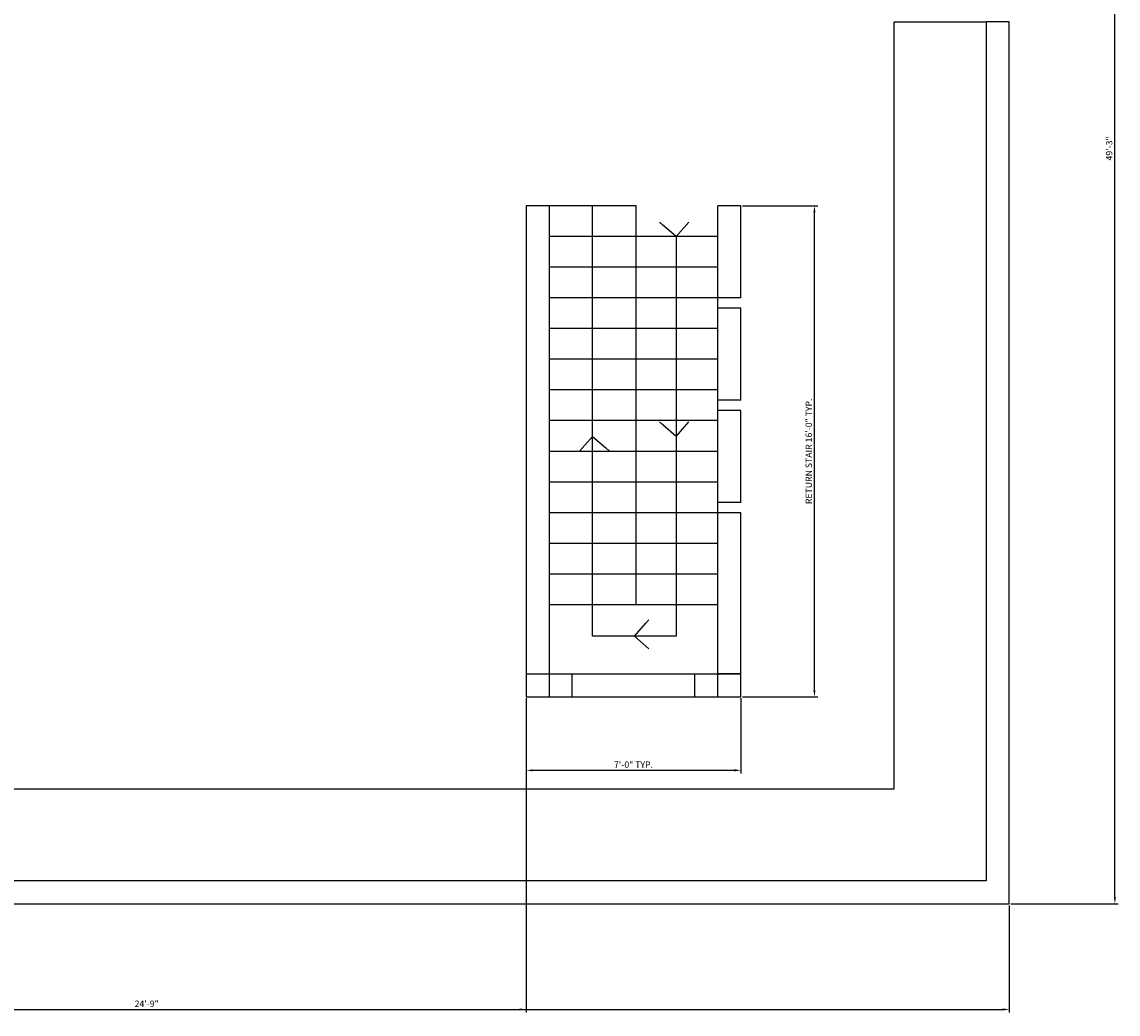
# Model space of a CAD drawing. Units: inches. Extents: x 250205121 to 250208111, y 89832590 to 89833271.
# Tile 3 of 14: x 250205601 to 250206030, y 89832590 to 89832978. Entities that reach past the tile are written whole.
import ezdxf

# ---------------------------------------------------------------- set-up
doc = ezdxf.new("R2010")
doc.units = ezdxf.units.IN
for name, color, linetype, lineweight in [('A-FLOR-STRS', 7, 'Continuous', 25), ('C-PROP', 8, 'Continuous', 25), ('dimensions', 2, 'Continuous', 18)]:
    doc.layers.add(name, color=color, linetype=linetype, lineweight=lineweight)
doc.styles.get("Standard").update_dxf_attribs({"font": 'arial.ttf'})
doc.dimstyles.new('ISO-25', dxfattribs={"dimtxt": 2.5, "dimasz": 2.5, "dimexe": 1.25, "dimexo": 0.625, "dimtad": 1, "dimlunit": 4, "dimtxsty": 'Standard', "dimcen": 2.5, "dimadec": 0, "dimazin": 0, "dimtfac": 1, "dimtmove": 0, "dimatfit": 3, "dimfxl": 1, "dimarcsym": 0})

# ---------------------------------------------------------------- blocks, each defined once
blk = doc.blocks.new('STAIR-RETURN')
for p, q in [((9, 192), (0, 192)), ((0, 192), (0, 0)), ((43, 192), (9, 192)), ((9, 192), (9, 0)), ((26, 23.7), (26, 192)), ((43, 36), (43, 192)), ((84, 192), (75, 192)), ((75, 0), (75, 192)), ((84, 156), (84, 192)), ((53.53, 184.53), (52.21, 185.69)), ((58.64, 180), (53.53, 184.53)), ((58.64, 180), (63.65, 185.66)), ((75, 180), (9, 180)), ((58.64, 180), (58.64, 23.7)), ((75, 168), (9, 168)), ((75, 156), (9, 156)), ((84, 156), (75, 156)), ((84, 152), (75, 152)), ((84, 116), (84, 152)), ((75, 144), (9, 144)), ((75, 132), (9, 132)), ((75, 120), (9, 120)), ((84, 116), (75, 116)), ((84, 112), (75, 112)), ((84, 76), (84, 112)), ((75, 108), (9, 108)), ((53.53, 106.37), (52.21, 107.54)), ((58.64, 101.85), (63.65, 107.51)), ((58.64, 101.85), (53.53, 106.37)), ((26, 101.85), (20.99, 96.18)), ((26, 101.85), (31.11, 97.32)), ((75, 96), (9, 96)), ((31.11, 97.32), (32.43, 96.16)), ((75, 84), (9, 84)), ((84, 76), (75, 76)), ((75, 72), (9, 72)), ((84, 72), (75, 72)), ((84, 0), (84, 72)), ((75, 60), (9, 60)), ((75, 48), (9, 48)), ((75, 36), (9, 36)), ((46.85, 28.81), (48.01, 30.12)), ((42.32, 23.7), (46.85, 28.81)), ((58.64, 23.7), (26, 23.7)), ((42.32, 23.7), (47.98, 18.68)), ((0, 9), (84, 9)), ((18, 0), (18, 9)), ((66, 0), (66, 9)), ((84, 9), (75, 9)), ((0, 0), (84, 0))]:
    blk.add_line(p, q)
blk = doc.blocks.new('*D37')
at = {"layer": 'Defpoints', "color": 0, "transparency": 16777216}
for p in [(250205881.91, 89832906.33), (250205910.71, 89832906.33), (250205881.91, 89832714.33)]:
    blk.add_point(p, dxfattribs=at)
at = {"layer": 'dimensions', "color": 0, "lineweight": -2, "transparency": 16777216}
for p, q in [((250205882.53, 89832906.33), (250205911.96, 89832906.33)), ((250205910.71, 89832716.83), (250205910.71, 89832903.83)), ((250205882.53, 89832714.33), (250205911.96, 89832714.33))]:
    blk.add_line(p, q, dxfattribs=at)
at = {"layer": 'dimensions', "color": 0, "transparency": 16777216}
for points in [[(250205910.29, 89832903.83), (250205911.12, 89832903.83), (250205910.71, 89832906.33)], [(250205910.29, 89832716.83), (250205911.12, 89832716.83), (250205910.71, 89832714.33)]]:
    blk.add_solid(points, dxfattribs=at)
at = {"layer": 'dimensions', "color": 0, "transparency": 16777216, "insert": (250205908.79, 89832810.33), "char_height": 2.5, "attachment_point": 5, "rotation": 90}
blk.add_mtext('RETURN STAIR 16\'-0" TYP.', dxfattribs=at)
blk = doc.blocks.new('*D38')
at = {"layer": 'Defpoints', "color": 0, "transparency": 16777216}
for p in [(250205797.91, 89832714.33), (250205881.91, 89832714.33), (250205881.91, 89832685.53)]:
    blk.add_point(p, dxfattribs=at)
at = {"layer": 'dimensions', "color": 0, "lineweight": -2, "transparency": 16777216}
for p, q in [((250205797.91, 89832713.7), (250205797.91, 89832684.28)), ((250205881.91, 89832713.7), (250205881.91, 89832684.28)), ((250205800.41, 89832685.53), (250205879.41, 89832685.53))]:
    blk.add_line(p, q, dxfattribs=at)
at = {"layer": 'dimensions', "color": 0, "transparency": 16777216}
for points in [[(250205800.41, 89832685.94), (250205800.41, 89832685.11), (250205797.91, 89832685.53)], [(250205879.41, 89832685.94), (250205879.41, 89832685.11), (250205881.91, 89832685.53)]]:
    blk.add_solid(points, dxfattribs=at)
at = {"layer": 'dimensions', "color": 0, "transparency": 16777216, "insert": (250205839.91, 89832687.43), "char_height": 2.5, "attachment_point": 5}
blk.add_mtext('7\'-0" TYP.', dxfattribs=at)
blk = doc.blocks.new('*D41')
at = {"layer": 'Defpoints', "color": 0, "transparency": 16777216}
for p in [(250205166.41, 89832633.33), (250205986.91, 89832633.33), (250205986.91, 89832591.98)]:
    blk.add_point(p, dxfattribs=at)
at = {"layer": 'dimensions', "color": 0, "lineweight": -2, "transparency": 16777216}
for p, q in [((250205166.41, 89832632.7), (250205166.41, 89832590.73)), ((250205986.91, 89832632.7), (250205986.91, 89832590.73)), ((250205168.91, 89832591.98), (250205984.41, 89832591.98))]:
    blk.add_line(p, q, dxfattribs=at)
at = {"layer": 'dimensions', "color": 0, "transparency": 16777216}
for points in [[(250205168.91, 89832592.39), (250205168.91, 89832591.56), (250205166.41, 89832591.98)], [(250205984.41, 89832592.39), (250205984.41, 89832591.56), (250205986.91, 89832591.98)]]:
    blk.add_solid(points, dxfattribs=at)
at = {"layer": 'dimensions', "color": 0, "transparency": 16777216, "insert": (250205576.66, 89832593.9), "char_height": 2.5, "attachment_point": 5}
blk.add_mtext('68\'-4 1/2"', dxfattribs=at)
blk = doc.blocks.new('*D42')
at = {"layer": 'Defpoints', "color": 0, "transparency": 16777216}
for p in [(250205986.91, 89833224.33), (250206028.26, 89833224.33), (250205986.91, 89832633.33)]:
    blk.add_point(p, dxfattribs=at)
at = {"layer": 'dimensions', "color": 0, "lineweight": -2, "transparency": 16777216}
for p, q in [((250205987.53, 89833224.33), (250206029.51, 89833224.33)), ((250206028.26, 89832635.83), (250206028.26, 89833221.83)), ((250205987.53, 89832633.33), (250206029.51, 89832633.33))]:
    blk.add_line(p, q, dxfattribs=at)
at = {"layer": 'dimensions', "color": 0, "transparency": 16777216}
for points in [[(250206027.84, 89833221.83), (250206028.67, 89833221.83), (250206028.26, 89833224.33)], [(250206027.84, 89832635.83), (250206028.67, 89832635.83), (250206028.26, 89832633.33)]]:
    blk.add_solid(points, dxfattribs=at)
at = {"layer": 'dimensions', "color": 0, "transparency": 16777216, "insert": (250206026.36, 89832928.83), "char_height": 2.5, "attachment_point": 5, "rotation": 90}
blk.add_mtext('49\'-3"', dxfattribs=at)
blk = doc.blocks.new('*D47')
at = {"layer": 'Defpoints', "color": 0, "transparency": 16777216}
for p in [(250205500.91, 89832714.33), (250205797.91, 89832714.33), (250205797.91, 89832591.98)]:
    blk.add_point(p, dxfattribs=at)
at = {"layer": 'dimensions', "color": 0, "lineweight": -2, "transparency": 16777216}
for p, q in [((250205500.91, 89832713.7), (250205500.91, 89832590.73)), ((250205797.91, 89832713.7), (250205797.91, 89832590.73)), ((250205503.41, 89832591.98), (250205795.41, 89832591.98))]:
    blk.add_line(p, q, dxfattribs=at)
at = {"layer": 'dimensions', "color": 0, "transparency": 16777216}
for points in [[(250205503.41, 89832592.39), (250205503.41, 89832591.56), (250205500.91, 89832591.98)], [(250205795.41, 89832592.39), (250205795.41, 89832591.56), (250205797.91, 89832591.98)]]:
    blk.add_solid(points, dxfattribs=at)
at = {"layer": 'dimensions', "color": 0, "transparency": 16777216, "insert": (250205649.41, 89832593.88), "char_height": 2.5, "attachment_point": 5}
blk.add_mtext('24\'-9"', dxfattribs=at)

msp = doc.modelspace()

# ---------------------------------------------------------------- linework, layer by layer
at = {"layer": 'C-PROP'}
for p, q in [((250205941.908, 89832678.328), (250205941.908, 89832978.328)), ((250205941.908, 89832978.328), (250205977.908, 89832978.328)), ((250205977.908, 89832978.328), (250205977.908, 89832978.328)), ((250205977.908, 89832978.328), (250205977.908, 89832642.328)), ((250205986.908, 89832978.328), (250205977.908, 89832978.328)), ((250205986.908, 89832633.328), (250205986.908, 89832978.328)), ((250205500.908, 89832678.328), (250205941.908, 89832678.328)), ((250205977.908, 89832642.328), (250205500.908, 89832642.328)), ((250205500.908, 89832633.328), (250205977.908, 89832633.328)), ((250205977.908, 89832633.328), (250205986.908, 89832633.328))]:
    msp.add_line(p, q, dxfattribs=at)

# ---------------------------------------------------------------- block references
at = {"layer": 'A-FLOR-STRS'}
msp.add_blockref('STAIR-RETURN', (250205797.908, 89832714.328), dxfattribs=at)

# ---------------------------------------------------------------- dimensions: what is measured, and where the dimension line sits
at = {"layer": 'dimensions'}
dim = msp.add_linear_dim(base=(250206028.258, 89833224.328), p1=(250205986.908, 89832633.328), p2=(250205986.908, 89833224.328), angle=90, dimstyle='ISO-25', override={"dimdec": 1, "dimlfac": 1, "dimrnd": 0, "dimzin": 1, "dimdsep": 46, "dimlunit": 4, "dimfrac": 2}, dxfattribs=at)
dim.commit()
dim.dimension.update_dxf_attribs({"geometry": '*D42', "text_midpoint": (250206026.355, 89832928.828)})
dim = msp.add_linear_dim(base=(250205910.708, 89832906.328), p1=(250205881.908, 89832714.328), p2=(250205881.908, 89832906.328), angle=90, text='RETURN STAIR <> TYP.', dimstyle='ISO-25', override={"dimdec": 1, "dimlfac": 1, "dimrnd": 0, "dimzin": 1, "dimdsep": 46, "dimlunit": 4, "dimfrac": 2}, dxfattribs=at)
dim.commit()
dim.dimension.update_dxf_attribs({"geometry": '*D37', "text_midpoint": (250205908.79, 89832810.328)})
for base, p1, p2, picture, middle in [((250205797.908, 89832591.978), (250205500.908, 89832714.328), (250205797.908, 89832714.328), '*D47', (250205649.408, 89832593.879)), ((250205986.908, 89832591.978), (250205166.408, 89832633.328), (250205986.908, 89832633.328), '*D41', (250205576.658, 89832593.896))]:
    dim = msp.add_linear_dim(base=base, p1=p1, p2=p2, dimstyle='ISO-25', override={"dimdec": 1, "dimlfac": 1, "dimrnd": 0, "dimzin": 1, "dimdsep": 46, "dimlunit": 4, "dimfrac": 2}, dxfattribs=at)
    dim.commit()
    dim.dimension.update_dxf_attribs({"geometry": picture, "text_midpoint": middle})
dim = msp.add_linear_dim(base=(250205881.908, 89832685.528), p1=(250205797.908, 89832714.328), p2=(250205881.908, 89832714.328), text='<> TYP.', dimstyle='ISO-25', override={"dimdec": 1, "dimlfac": 1, "dimrnd": 0, "dimzin": 1, "dimdsep": 46, "dimlunit": 4, "dimfrac": 2}, dxfattribs=at)
dim.commit()
dim.dimension.update_dxf_attribs({"geometry": '*D38', "text_midpoint": (250205839.908, 89832687.429)})

doc.saveas('drawing.dxf')
